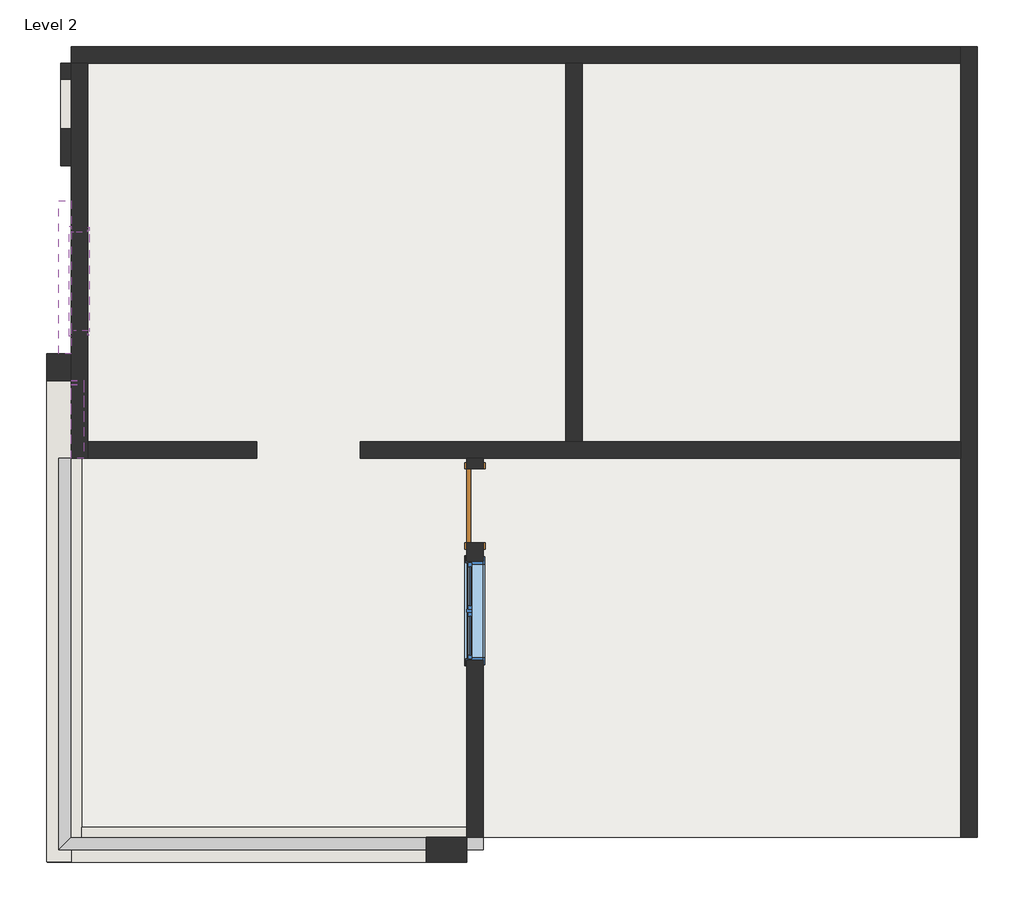
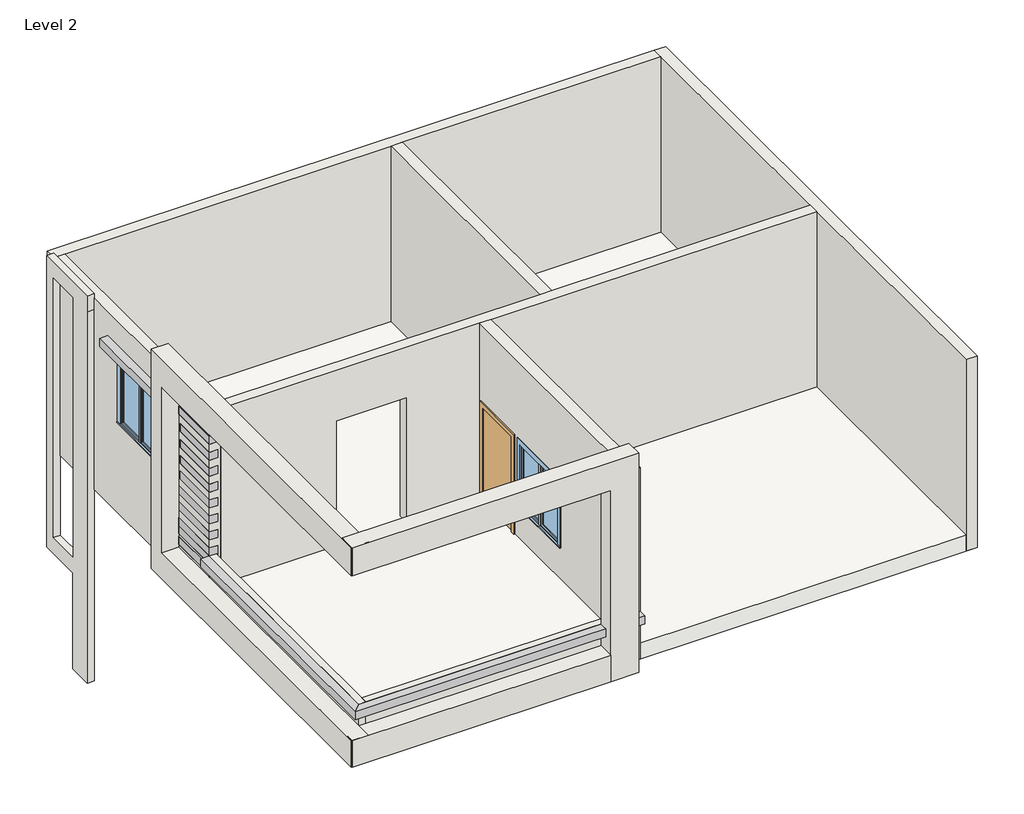
# One storey, incomplete: 14 proxies, 10 walls, 2 windows, 1 door, 1 roof.
"""IFC4 building model written with IfcOpenShell, lengths in millimetres."""

from ifc_helpers import new_model, si_unit, frame, origin, place, context, project, spatial, polyline, outline, extrude, faceted_brep, transform, mapped, element, save
from components import door_54dd4da4, walls_1_walls_1_33573b5d, window_0862ab64

model = new_model("IFC4")

# Units and contexts
model_context = context("Model", 3, world=origin())
ifc_project = project(units=[si_unit("LENGTHUNIT", "METRE", prefix="MILLI")], contexts=[model_context])

# Site, building, storey
site = spatial("IfcSite", under=ifc_project)
building = spatial("IfcBuilding", under=site)
storey = spatial("IfcBuildingStorey", under=building, Name="Level 2", Elevation=3657.6)

# Proxies
placement = place(None, origin())
element("IfcBuildingElementProxy", 1, Name="Cornice", ObjectType="Cornice", at=placement, inside=storey, context=model_context, shape_type="SweptSolid", body=[
    extrude(outline(polyline([(-12556.4681702, 5517.1742715), (-12708.8681702, 5517.1742715), (-12708.8681702, 7399.8573992), (-12556.4681702, 7399.8573992), (-12556.4681702, 5517.1742715)])), frame((0.0, 0.0, 6705.6), z_axis=(0.0, 0.0, 1.0), x_axis=(1.0, 0.0, 0.0)), (0.0, 0.0, 1.0), 152.4),
])
element("IfcBuildingElementProxy", 2, Name="Cornice", ObjectType="Cornice", at=placement, inside=storey, context=model_context, shape_type="SweptSolid", body=[
    extrude(outline(polyline([(-12708.8681702, 4224.2612165), (-12556.4681702, 4224.2612165), (-12556.4681702, -449.3387835), (-12708.8681702, -601.7387835), (-12708.8681702, 4224.2612165)])), frame((0.0, 0.0, 4419.6), z_axis=(0.0, 0.0, 1.0), x_axis=(1.0, 0.0, 0.0)), (0.0, 0.0, 1.0), 152.4),
])
element("IfcBuildingElementProxy", 3, Name="Cornice", ObjectType="Cornice", at=placement, inside=storey, context=model_context, shape_type="SweptSolid", body=[
    extrude(outline(polyline([(-12708.8681702, -601.7387835), (-12556.4681702, -449.3387835), (-7476.4681702, -449.3387835), (-7476.4681702, -601.7387835), (-12708.8681702, -601.7387835)])), frame((0.0, 0.0, 4419.6), z_axis=(0.0, 0.0, 1.0), x_axis=(1.0, 0.0, 0.0)), (0.0, 0.0, 1.0), 152.4),
])
element("IfcBuildingElementProxy", 4, Name="Reveal", ObjectType="Reveal", at=placement, inside=storey, context=model_context, shape_type="SweptSolid", body=[
    extrude(outline(polyline([(-12404.0681702, 4224.2612165), (-12556.4681702, 4224.2612165), (-12556.4681702, 5180.9930334), (-12404.0681702, 5180.9930334), (-12404.0681702, 4224.2612165)])), frame((0.0, 0.0, 7010.4), z_axis=(0.0, 0.0, 1.0), x_axis=(1.0, 0.0, 0.0)), (0.0, 0.0, 1.0), 152.4),
])
element("IfcBuildingElementProxy", 5, Name="Reveal", ObjectType="Reveal", at=placement, inside=storey, context=model_context, shape_type="SweptSolid", body=[
    extrude(outline(polyline([(-12404.0681702, 4224.2612165), (-12556.4681702, 4224.2612165), (-12556.4681702, 5180.9930334), (-12404.0681702, 5180.9930334), (-12404.0681702, 4224.2612165)])), frame((0.0, 0.0, 6705.6), z_axis=(0.0, 0.0, 1.0), x_axis=(1.0, 0.0, 0.0)), (0.0, 0.0, 1.0), 152.4),
])
element("IfcBuildingElementProxy", 6, Name="Reveal", ObjectType="Reveal", at=placement, inside=storey, context=model_context, shape_type="SweptSolid", body=[
    extrude(outline(polyline([(-12404.0681702, 4224.2612165), (-12556.4681702, 4224.2612165), (-12556.4681702, 5130.1930334), (-12404.0681702, 5130.1930334), (-12404.0681702, 4224.2612165)])), frame((0.0, 0.0, 6400.8), z_axis=(0.0, 0.0, 1.0), x_axis=(1.0, 0.0, 0.0)), (0.0, 0.0, 1.0), 152.4),
])
element("IfcBuildingElementProxy", 7, Name="Reveal", ObjectType="Reveal", at=placement, inside=storey, context=model_context, shape_type="SweptSolid", body=[
    extrude(outline(polyline([(-12404.0681702, 4224.2612165), (-12556.4681702, 4224.2612165), (-12556.4681702, 5130.1930334), (-12404.0681702, 5130.1930334), (-12404.0681702, 4224.2612165)])), frame((0.0, 0.0, 6096.0), z_axis=(0.0, 0.0, 1.0), x_axis=(1.0, 0.0, 0.0)), (0.0, 0.0, 1.0), 152.4),
])
element("IfcBuildingElementProxy", 8, Name="Reveal", ObjectType="Reveal", at=placement, inside=storey, context=model_context, shape_type="SweptSolid", body=[
    extrude(outline(polyline([(-12404.0681702, 4224.2612165), (-12556.4681702, 4224.2612165), (-12556.4681702, 5130.1930334), (-12404.0681702, 5130.1930334), (-12404.0681702, 4224.2612165)])), frame((0.0, 0.0, 5791.2), z_axis=(0.0, 0.0, 1.0), x_axis=(1.0, 0.0, 0.0)), (0.0, 0.0, 1.0), 152.4),
])
element("IfcBuildingElementProxy", 9, Name="Reveal", ObjectType="Reveal", at=placement, inside=storey, context=model_context, shape_type="SweptSolid", body=[
    extrude(outline(polyline([(-12404.0681702, 4224.2612165), (-12556.4681702, 4224.2612165), (-12556.4681702, 5138.6612165), (-12404.0681702, 5138.6612165), (-12404.0681702, 4224.2612165)])), frame((0.0, 0.0, 5486.4), z_axis=(0.0, 0.0, 1.0), x_axis=(1.0, 0.0, 0.0)), (0.0, 0.0, 1.0), 152.4),
])
element("IfcBuildingElementProxy", 10, Name="Reveal", ObjectType="Reveal", at=placement, inside=storey, context=model_context, shape_type="SweptSolid", body=[
    extrude(outline(polyline([(-12404.0681702, 4224.2612165), (-12556.4681702, 4224.2612165), (-12556.4681702, 5189.4612165), (-12404.0681702, 5189.4612165), (-12404.0681702, 4224.2612165)])), frame((0.0, 0.0, 5181.6), z_axis=(0.0, 0.0, 1.0), x_axis=(1.0, 0.0, 0.0)), (0.0, 0.0, 1.0), 152.4),
])
element("IfcBuildingElementProxy", 11, Name="Reveal", ObjectType="Reveal", at=placement, inside=storey, context=model_context, shape_type="SweptSolid", body=[
    extrude(outline(polyline([(-12404.0681702, 4224.2612165), (-12556.4681702, 4224.2612165), (-12556.4681702, 5189.4612165), (-12404.0681702, 5189.4612165), (-12404.0681702, 4224.2612165)])), frame((0.0, 0.0, 4876.8), z_axis=(0.0, 0.0, 1.0), x_axis=(1.0, 0.0, 0.0)), (0.0, 0.0, 1.0), 152.4),
])
element("IfcBuildingElementProxy", 12, Name="Reveal", ObjectType="Reveal", at=placement, inside=storey, context=model_context, shape_type="SweptSolid", body=[
    extrude(outline(polyline([(-12404.0681702, 4224.2612165), (-12556.4681702, 4224.2612165), (-12556.4681702, 5180.9930334), (-12404.0681702, 5180.9930334), (-12404.0681702, 4224.2612165)])), frame((0.0, 0.0, 4572.0), z_axis=(0.0, 0.0, 1.0), x_axis=(1.0, 0.0, 0.0)), (0.0, 0.0, 1.0), 152.4),
])
element("IfcBuildingElementProxy", 13, Name="Reveal", ObjectType="Reveal", at=placement, inside=storey, context=model_context, shape_type="SweptSolid", body=[
    extrude(outline(polyline([(-12404.0681702, 4224.2612165), (-12556.4681702, 4224.2612165), (-12556.4681702, 5180.9930334), (-12404.0681702, 5180.9930334), (-12404.0681702, 4224.2612165)])), frame((0.0, 0.0, 4419.6), z_axis=(0.0, 0.0, 1.0), x_axis=(1.0, 0.0, 0.0)), (0.0, 0.0, 1.0), 152.4),
])
element("IfcBuildingElementProxy", 14, Name="Reveal", ObjectType="Reveal", at=placement, inside=storey, context=model_context, shape_type="SweptSolid", body=[
    extrude(outline(polyline([(-12404.0681702, 4224.2612165), (-12556.4681702, 4224.2612165), (-12556.4681702, 5180.9930334), (-12404.0681702, 5180.9930334), (-12404.0681702, 4224.2612165)])), frame((0.0, 0.0, 4216.4), z_axis=(0.0, 0.0, 1.0), x_axis=(1.0, 0.0, 0.0)), (0.0, 0.0, 1.0), 152.4),
])

# Door
door_shape = door_54dd4da4(model_context)
element("IfcDoor", 15, ObjectType="Single-Flush : 36\" x 84\"", at=placement, inside=storey, context=model_context, shape_type="MappedRepresentation", body=[
    mapped(door_shape, transform((-7578.0681702, 3640.0612165, 3657.6), x_axis=(0.0, 1.0, 0.0), y_axis=(-1.0, 0.0, 0.0), z_axis=(0.0, 0.0, 1.0))),
])

# Roof
element("IfcRoof", 16, ObjectType="Generic - 12\"", at=placement, inside=storey, context=model_context, shape_type="SweptSolid", body=[
    extrude(outline(polyline([(-12556.4681702, 9304.2612165), (-1380.4681702, 9304.2612165), (-1380.4681702, -449.3387835), (-12556.4681702, -449.3387835), (-12556.4681702, 9304.2612165)])), frame((0.0, 0.0, 3657.6), z_axis=(0.0, 0.0, 1.0), x_axis=(1.0, 0.0, 0.0)), (0.0, 0.0, 1.0), 304.8),
])

# Walls
element("IfcWall", 17, ObjectType="Generic - 5\"", at=placement, inside=storey, context=model_context, shape_type="Brep", body=[
    faceted_brep([(-12556.4681702, 4224.2612165, 3962.4), (-12556.4681702, -449.3387835, 3962.4), (-12556.4681702, -449.3387835, 4572.0), (-12556.4681702, 4224.2612165, 4572.0), (-12556.4681702, 4224.2612165, 4419.6), (-12556.4681702, 4224.2612165, 4368.8), (-12556.4681702, 4224.2612165, 4216.4), (-12429.4681702, 4224.2612165, 3962.4), (-12429.4681702, 4224.2612165, 4572.0), (-12429.4681702, -322.3387835, 4572.0), (-12429.4681702, -449.3387835, 4572.0), (-12429.4681702, -449.3387835, 3962.4), (-12429.4681702, -322.3387835, 3962.4)], [[[0, 1, 2, 3, 4, 5, 6]], [[7, 8, 9, 10, 11, 12]], [[1, 0, 7, 12, 11]], [[3, 2, 10, 9, 8]], [[0, 6, 5, 4, 3, 8, 7]], [[2, 1, 11, 10]]]),
])
element("IfcWall", 18, ObjectType="Generic - 5\"", at=placement, inside=storey, context=model_context, shape_type="Brep", body=[
    faceted_brep([(-12429.4681702, -449.3387835, 3962.4), (-7679.6681702, -449.3387835, 3962.4), (-7679.6681702, -449.3387835, 4419.6), (-7679.6681702, -449.3387835, 4572.0), (-12429.4681702, -449.3387835, 4572.0), (-12429.4681702, -449.3387835, 4419.6), (-7679.6681702, -322.3387835, 3962.4), (-12429.4681702, -322.3387835, 3962.4), (-12429.4681702, -322.3387835, 4572.0), (-7679.6681702, -322.3387835, 4572.0)], [[[0, 1, 2, 3, 4, 5]], [[6, 7, 8, 9]], [[1, 0, 7, 6]], [[4, 3, 9, 8]], [[4, 8, 7, 0, 5]], [[1, 6, 9, 3, 2]]]),
])
element("IfcWall", 19, ObjectType="Generic - 5\"", at=placement, inside=storey, context=model_context, shape_type="SweptSolid", body=[
    extrude(outline(polyline([(7831.0612165, 0.0), (7831.0612165, 7094.0468042), (7831.0612165, 7398.8468042), (9101.0612165, 7398.8468042), (9101.0612165, 1828.8), (8288.2612165, 1828.8), (8288.2612165, 0.0), (7831.0612165, 0.0)]), holes=[polyline([(8897.8612165, 2133.6), (8897.8612165, 7094.0468042), (8288.2612165, 7094.0468042), (8288.2612165, 2133.6), (8897.8612165, 2133.6)])]), frame((-12683.4681702, 0.0, 0.0), z_axis=(1.0, 0.0, 0.0), x_axis=(0.0, 1.0, 0.0)), (0.0, 0.0, 1.0), 127.0),
])
element("IfcWall", 20, ObjectType="Generic - 8\"", at=placement, inside=storey, context=model_context, shape_type="Brep", body=[
    faceted_brep([(-12556.4681702, 9101.0612165, 3657.6), (-12353.2681702, 9101.0612165, 3657.6), (-6460.4681702, 9101.0612165, 3657.6), (-6257.2681702, 9101.0612165, 3657.6), (-1583.6681702, 9101.0612165, 3657.6), (-1583.6681702, 9101.0612165, 7315.2), (-6257.2681702, 9101.0612165, 7315.2), (-6460.4681702, 9101.0612165, 7315.2), (-12353.2681702, 9101.0612165, 7315.2), (-12556.4681702, 9101.0612165, 7315.2), (-12556.4681702, 9304.2612165, 3657.6), (-12556.4681702, 9304.2612165, 7315.2), (-1583.6681702, 9304.2612165, 7315.2), (-1583.6681702, 9304.2612165, 3657.6)], [[[0, 1, 2, 3, 4, 5, 6, 7, 8, 9]], [[10, 11, 12, 13]], [[4, 3, 2, 1, 0, 10, 13]], [[9, 8, 7, 6, 5, 12, 11]], [[0, 9, 11, 10]], [[5, 4, 13, 12]]]),
])
element("IfcWall", 21, ObjectType="Generic - 8\"", at=placement, inside=storey, context=model_context, shape_type="Brep", body=[
    faceted_brep([(-12353.2681702, 4224.2612165, 3657.6), (-12353.2681702, 4427.4612165, 3657.6), (-12353.2681702, 9101.0612165, 3657.6), (-12353.2681702, 9101.0612165, 7315.2), (-12353.2681702, 4427.4612165, 7315.2), (-12353.2681702, 4224.2612165, 7315.2), (-12353.2681702, 7018.2612165, 6617.6597463), (-12353.2681702, 7018.2612165, 5398.4597463), (-12353.2681702, 5799.0612165, 5398.4597463), (-12353.2681702, 5799.0612165, 6617.6597463), (-12556.4681702, 9101.0612165, 3657.6), (-12556.4681702, 4224.2612165, 3657.6), (-12556.4681702, 4224.2612165, 3962.4), (-12556.4681702, 4224.2612165, 4216.4), (-12556.4681702, 5180.9930334, 4216.4), (-12556.4681702, 5180.9930334, 4368.8), (-12556.4681702, 4224.2612165, 4368.8), (-12556.4681702, 4224.2612165, 4419.6), (-12556.4681702, 5180.9930334, 4419.6), (-12556.4681702, 5180.9930334, 4724.4), (-12556.4681702, 4224.2612165, 4724.4), (-12556.4681702, 4224.2612165, 4876.8), (-12556.4681702, 5189.4612165, 4876.8), (-12556.4681702, 5189.4612165, 5029.2), (-12556.4681702, 4224.2612165, 5029.2), (-12556.4681702, 4224.2612165, 5181.6), (-12556.4681702, 5189.4612165, 5181.6), (-12556.4681702, 5189.4612165, 5334.0), (-12556.4681702, 4224.2612165, 5334.0), (-12556.4681702, 4224.2612165, 5486.4), (-12556.4681702, 5138.6612165, 5486.4), (-12556.4681702, 5138.6612165, 5638.8), (-12556.4681702, 4224.2612165, 5638.8), (-12556.4681702, 4224.2612165, 5791.2), (-12556.4681702, 5130.1930334, 5791.2), (-12556.4681702, 5130.1930334, 5943.6), (-12556.4681702, 4224.2612165, 5943.6), (-12556.4681702, 4224.2612165, 6096.0), (-12556.4681702, 5130.1930334, 6096.0), (-12556.4681702, 5130.1930334, 6248.4), (-12556.4681702, 4224.2612165, 6248.4), (-12556.4681702, 4224.2612165, 6400.8), (-12556.4681702, 5130.1930334, 6400.8), (-12556.4681702, 5130.1930334, 6553.2), (-12556.4681702, 4224.2612165, 6553.2), (-12556.4681702, 4224.2612165, 6705.6), (-12556.4681702, 5180.9930334, 6705.6), (-12556.4681702, 5180.9930334, 6858.0), (-12556.4681702, 4224.2612165, 6858.0), (-12556.4681702, 4224.2612165, 7010.4), (-12556.4681702, 5180.9930334, 7010.4), (-12556.4681702, 5180.9930334, 7162.8), (-12556.4681702, 4224.2612165, 7162.8), (-12556.4681702, 4224.2612165, 7315.2), (-12556.4681702, 9101.0612165, 7315.2), (-12556.4681702, 7018.2612165, 5398.4597463), (-12556.4681702, 7018.2612165, 6617.6597463), (-12556.4681702, 5799.0612165, 6617.6597463), (-12556.4681702, 5799.0612165, 5398.4597463), (-12404.0681702, 4224.2612165, 7162.8), (-12404.0681702, 4224.2612165, 7010.4), (-12404.0681702, 4224.2612165, 6858.0), (-12404.0681702, 4224.2612165, 6705.6), (-12404.0681702, 4224.2612165, 6553.2), (-12404.0681702, 4224.2612165, 6400.8), (-12404.0681702, 4224.2612165, 6248.4), (-12404.0681702, 4224.2612165, 6096.0), (-12404.0681702, 4224.2612165, 5943.6), (-12404.0681702, 4224.2612165, 5791.2), (-12404.0681702, 4224.2612165, 5638.8), (-12404.0681702, 4224.2612165, 5486.4), (-12404.0681702, 4224.2612165, 5334.0), (-12404.0681702, 4224.2612165, 5181.6), (-12404.0681702, 4224.2612165, 5029.2), (-12404.0681702, 4224.2612165, 4876.8), (-12404.0681702, 4224.2612165, 4724.4), (-12404.0681702, 4224.2612165, 4419.6), (-12404.0681702, 4224.2612165, 4368.8), (-12404.0681702, 4224.2612165, 4216.4), (-12404.0681702, 5180.9930334, 7010.4), (-12404.0681702, 5180.9930334, 7162.8), (-12404.0681702, 5180.9930334, 6705.6), (-12404.0681702, 5180.9930334, 6858.0), (-12404.0681702, 5189.4612165, 5181.6), (-12404.0681702, 5189.4612165, 5334.0), (-12404.0681702, 5189.4612165, 4876.8), (-12404.0681702, 5189.4612165, 5029.2), (-12404.0681702, 5180.9930334, 4724.4), (-12404.0681702, 5180.9930334, 4419.6), (-12404.0681702, 5180.9930334, 4216.4), (-12404.0681702, 5180.9930334, 4368.8), (-12404.0681702, 5130.1930334, 6553.2), (-12404.0681702, 5130.1930334, 6400.8), (-12404.0681702, 5130.1930334, 6248.4), (-12404.0681702, 5130.1930334, 6096.0), (-12404.0681702, 5130.1930334, 5943.6), (-12404.0681702, 5130.1930334, 5791.2), (-12404.0681702, 5138.6612165, 5638.8), (-12404.0681702, 5138.6612165, 5486.4)], [[[0, 1, 2, 3, 4, 5], [6, 7, 8, 9]], [[10, 11, 12, 13, 14, 15, 16, 17, 18, 19, 20, 21, 22, 23, 24, 25, 26, 27, 28, 29, 30, 31, 32, 33, 34, 35, 36, 37, 38, 39, 40, 41, 42, 43, 44, 45, 46, 47, 48, 49, 50, 51, 52, 53, 54], [55, 56, 57, 58]], [[2, 1, 0, 11, 10]], [[5, 4, 3, 54, 53]], [[3, 2, 10, 54]], [[5, 53, 52, 59, 60, 49, 48, 61, 62, 45, 44, 63, 64, 41, 40, 65, 66, 37, 36, 67, 68, 33, 32, 69, 70, 29, 28, 71, 72, 25, 24, 73, 74, 21, 20, 75, 76, 17, 16, 77, 78, 13, 12, 11, 0]], [[79, 50, 49, 60]], [[79, 60, 59, 80]], [[80, 59, 52, 51]], [[81, 46, 45, 62]], [[81, 62, 61, 82]], [[82, 61, 48, 47]], [[83, 26, 25, 72]], [[83, 72, 71, 84]], [[84, 71, 28, 27]], [[85, 22, 21, 74]], [[85, 74, 73, 86]], [[86, 73, 24, 23]], [[75, 87, 88, 76]], [[87, 75, 20, 19]], [[88, 18, 17, 76]], [[89, 14, 13, 78]], [[90, 89, 78, 77]], [[15, 90, 77, 16]], [[90, 15, 14, 89]], [[87, 19, 18, 88]], [[22, 85, 86, 23]], [[26, 83, 84, 27]], [[46, 81, 82, 47]], [[50, 79, 80, 51]], [[7, 6, 56, 55]], [[8, 7, 55, 58]], [[9, 8, 58, 57]], [[6, 9, 57, 56]], [[91, 43, 42, 92]], [[92, 42, 41, 64]], [[91, 92, 64, 63]], [[43, 91, 63, 44]], [[93, 39, 38, 94]], [[94, 38, 37, 66]], [[93, 94, 66, 65]], [[39, 93, 65, 40]], [[95, 35, 34, 96]], [[96, 34, 33, 68]], [[95, 96, 68, 67]], [[35, 95, 67, 36]], [[97, 31, 30, 98]], [[98, 30, 29, 70]], [[97, 98, 70, 69]], [[31, 97, 69, 32]]]),
])
element("IfcWall", 22, ObjectType="Generic - 8\"", at=placement, inside=storey, context=model_context, shape_type="Brep", body=[
    faceted_brep([(-1583.6681702, 9304.2612165, 3657.6), (-1583.6681702, 9101.0612165, 3657.6), (-1583.6681702, 4427.4612165, 3657.6), (-1583.6681702, 4224.2612165, 3657.6), (-1583.6681702, -449.3387835, 3657.6), (-1583.6681702, -449.3387835, 7315.2), (-1583.6681702, 4224.2612165, 7315.2), (-1583.6681702, 4427.4612165, 7315.2), (-1583.6681702, 9101.0612165, 7315.2), (-1583.6681702, 9304.2612165, 7315.2), (-1380.4681702, 9304.2612165, 3657.6), (-1380.4681702, 9304.2612165, 7315.2), (-1380.4681702, -449.3387835, 7315.2), (-1380.4681702, -449.3387835, 3657.6)], [[[0, 1, 2, 3, 4, 5, 6, 7, 8, 9]], [[10, 11, 12, 13]], [[4, 3, 2, 1, 0, 10, 13]], [[9, 8, 7, 6, 5, 12, 11]], [[0, 9, 11, 10]], [[4, 13, 12, 5]]]),
])
element("IfcWall", 23, ObjectType="Generic - 8\"", at=placement, inside=storey, context=model_context, shape_type="Brep", body=[
    faceted_brep([(-7679.6681702, 4224.2612165, 3657.6), (-7679.6681702, 4097.2612165, 3657.6), (-7679.6681702, 4097.2612165, 5791.2), (-7679.6681702, 3182.8612165, 5791.2), (-7679.6681702, 3182.8612165, 3657.6), (-7679.6681702, -449.3387835, 3657.6), (-7679.6681702, -449.3387835, 3962.4), (-7679.6681702, -449.3387835, 4572.0), (-7679.6681702, -449.3387835, 7315.2), (-7679.6681702, 2954.2612165, 7315.2), (-7679.6681702, 3868.6612165, 7315.2), (-7679.6681702, 4224.2612165, 7315.2), (-7679.6681702, 2954.2612165, 5791.2), (-7679.6681702, 1735.0612165, 5791.2), (-7679.6681702, 1735.0612165, 4572.0), (-7679.6681702, 2954.2612165, 4572.0), (-7476.4681702, 4097.2612165, 5791.2), (-7476.4681702, 4097.2612165, 3657.6), (-7476.4681702, 4224.2612165, 3657.6), (-7476.4681702, 4224.2612165, 7315.2), (-7476.4681702, 3868.6612165, 7315.2), (-7476.4681702, 2954.2612165, 7315.2), (-7476.4681702, -449.3387835, 7315.2), (-7476.4681702, -449.3387835, 3657.6), (-7476.4681702, 3182.8612165, 3657.6), (-7476.4681702, 3182.8612165, 5791.2), (-7476.4681702, 2954.2612165, 5791.2), (-7476.4681702, 2954.2612165, 4572.0), (-7476.4681702, 1735.0612165, 4572.0), (-7476.4681702, 1735.0612165, 5791.2)], [[[0, 1, 2, 3, 4, 5, 6, 7, 8, 9, 10, 11], [12, 13, 14, 15]], [[16, 17, 18, 19, 20, 21, 22, 23, 24, 25], [26, 27, 28, 29]], [[18, 17, 1, 0]], [[24, 23, 5, 4]], [[11, 10, 9, 8, 22, 21, 20, 19]], [[0, 11, 19, 18]], [[5, 23, 22, 8, 7, 6]], [[27, 26, 12, 15]], [[28, 27, 15, 14]], [[29, 28, 14, 13]], [[26, 29, 13, 12]], [[2, 1, 17, 16]], [[3, 2, 16, 25]], [[4, 3, 25, 24]]]),
])
element("IfcWall", 24, ObjectType="Generic - 8\"", at=placement, inside=storey, context=model_context, shape_type="Brep", body=[
    faceted_brep([(-12353.2681702, 4224.2612165, 7315.2), (-12353.2681702, 4224.2612165, 3657.6), (-10267.8388214, 4224.2612165, 3657.6), (-10267.8388214, 4224.2612165, 6351.2959794), (-8991.5303488, 4224.2612165, 6351.2959794), (-8991.5303488, 4224.2612165, 3657.6), (-7679.6681702, 4224.2612165, 3657.6), (-7476.4681702, 4224.2612165, 3657.6), (-1583.6681702, 4224.2612165, 3657.6), (-1583.6681702, 4224.2612165, 7315.2), (-7476.4681702, 4224.2612165, 7315.2), (-7679.6681702, 4224.2612165, 7315.2), (-12353.2681702, 4427.4612165, 3657.6), (-12353.2681702, 4427.4612165, 7315.2), (-6460.4681702, 4427.4612165, 7315.2), (-6257.2681702, 4427.4612165, 7315.2), (-1583.6681702, 4427.4612165, 7315.2), (-1583.6681702, 4427.4612165, 3657.6), (-6257.2681702, 4427.4612165, 3657.6), (-6460.4681702, 4427.4612165, 3657.6), (-8991.5303488, 4427.4612165, 3657.6), (-8991.5303488, 4427.4612165, 6351.2959794), (-10267.8388214, 4427.4612165, 6351.2959794), (-10267.8388214, 4427.4612165, 3657.6)], [[[0, 1, 2, 3, 4, 5, 6, 7, 8, 9, 10, 11]], [[12, 13, 14, 15, 16, 17, 18, 19, 20, 21, 22, 23]], [[9, 8, 17, 16]], [[0, 13, 12, 1]], [[0, 11, 10, 9, 16, 15, 14, 13]], [[5, 4, 21, 20]], [[3, 2, 23, 22]], [[4, 3, 22, 21]], [[2, 1, 12, 23]], [[8, 7, 6, 5, 20, 19, 18, 17]]]),
])
element("IfcWall", 25, ObjectType="Generic - 8\"", at=placement, inside=storey, context=model_context, shape_type="SweptSolid", body=[
    extrude(outline(polyline([(-6460.4681702, 4427.4612165), (-6460.4681702, 9101.0612165), (-6257.2681702, 9101.0612165), (-6257.2681702, 4427.4612165), (-6460.4681702, 4427.4612165)])), frame((0.0, 0.0, 3657.6), z_axis=(0.0, 0.0, 1.0), x_axis=(1.0, 0.0, 0.0)), (0.0, 0.0, 1.0), 3657.6),
])
walls_1_walls_1_shape = walls_1_walls_1_33573b5d(model_context)
element("IfcWall", 26, ObjectType="Walls 1 : Walls 1", at=placement, inside=storey, context=model_context, shape_type="MappedRepresentation", body=[
    mapped(walls_1_walls_1_shape, transform((0.0, 0.0, 0.0), x_axis=(1.0, 0.0, 0.0), y_axis=(0.0, 1.0, 0.0), z_axis=(0.0, 0.0, 1.0))),
])

# Windows
window_shape = window_0862ab64(model_context)
element("IfcWindow", 27, ObjectType="Casement Dbl with Trim : 48\" x 48\"", at=placement, inside=storey, context=model_context, shape_type="MappedRepresentation", body=[
    mapped(window_shape, transform((-12435.8181702, 6408.6612165, 4484.0597463), x_axis=(0.0, 1.0, 0.0), y_axis=(-1.0, 0.0, 0.0), z_axis=(0.0, 0.0, 1.0))),
])
element("IfcWindow", 28, ObjectType="Casement Dbl with Trim : 48\" x 48\"", at=placement, inside=storey, context=model_context, shape_type="MappedRepresentation", body=[
    mapped(window_shape, transform((-7559.0181702, 2344.6612165, 3657.6), x_axis=(0.0, 1.0, 0.0), y_axis=(-1.0, 0.0, 0.0), z_axis=(0.0, 0.0, 1.0))),
])

save(model, "model.ifc")

# Revit data of these elements
# Type "Single-Flush : 36\" x 84\""
#   Type Mark = "1"
#   Construction Type Id = "MDOOR"
#   Assembly Code = "C1020"
#   Analytic Construction = "Metal"
#   Thickness = 0' - 2"
#   Heat Transfer Coefficient (U) = 0.651978 BTU/(h·ft²·°F)
#   Height = 7' - 0"
#   Trim Projection Ext = 0' - 1"
#   Trim Projection Int = 0' - 1"
#   Trim Width = 0' - 3"
#   Width = 3' - 0"
#   Define Thermal Properties by = 1
#   Door Material = Door - Panel
#   Frame Material = Door - Frame
#   Visual Light Transmittance = 0
#   Solar Heat Gain Coefficient = 0
#   Function = (empty or 0)
#   Wall Closure = (empty or 0)
# Type "Generic - 12\""
#   Assembly Code = "B1020"
#   Layers, outside or top first: 1' - 0" no material (function 1)
# Type "Generic - 5\""
#   Assembly Code = "B2010"
#   Layers, outside or top first: 0' - 5" no material (function 1)
# Type "Generic - 8\""
#   Assembly Code = "B2010"
#   Layers, outside or top first: 0' - 8" no material (function 1)
# Type "Casement Dbl with Trim : 48\" x 48\""
#   Type Mark = "13"
#   Construction Type Id = "GSP4R"
#   Assembly Code = "B2020100"
#   Analytic Construction = "1/8 in Pilkington single glazing"
#   Visual Light Transmittance = 0.9
#   Solar Heat Gain Coefficient = 0.78
#   Heat Transfer Coefficient (U) = 0.6496 BTU/(h·ft²·°F)
#   Height = 4' - 0"
#   Default Sill Height = 3' - 0"
#   Trim Projection - Ext. = 0' - 0 1/2"
#   Trim Projection - Int. = 0' - 0 3/4"
#   Trim Width - Exterior = 0' - 3 1/2"
#   Trim Width - Interior = 0' - 3 1/2"
#   Width = 4' - 0"
#   Window Inset = 0' - 0 3/4"
#   Define Thermal Properties by = 1
#   Glass Pane Material = Glass
#   Sash Material = Sash
#   Trim Exterior Material = Trim
#   Trim Interior Material = Trim
#   Wall Closure = (empty or 0)
# Elements 1, 2, 3 (IfcBuildingElementProxy, "Cornice")
#   Phase Created = New Construction
#   Materials on its faces: "Default Wall"
# Element 15 (IfcDoor, "Single-Flush : 36\" x 84\"")
#   Phase Created = New Construction
#   Materials on its faces: "Door - Frame", "Door - Panel"
# Element 16 (IfcRoof, "Generic - 12\"")
#   built-in parameter 1001705 = 13 (stored number, unit not read)
#   built-in parameter 1001710 = 33615
#   Phase Created = New Construction
#   Materials on its faces: "Default Roof"
# Elements 17, 18 (IfcWall, "Generic - 5\"")
#   built-in parameter 1001111 = 1' - 0"
#   Top Offset = -9' - 0"
#   Base Offset = 1' - 0"
#   wall height = 2' - 0"
#   Phase Created = New Construction
#   Base Constraint = Level 2
#   Top Constraint = Level 3
#   Materials on its faces: "Default Wall"
# Element 19 (IfcWall, "Generic - 5\"")
#   built-in parameter 1001111 = -12' - 0"
#   Top Offset = -0' - 8.70682"
#   Base Offset = -12' - 0"
#   wall height = 23' - 3.29318"
#   Phase Created = New Construction
#   Base Constraint = Level 2
#   Top Constraint = Level 3
#   Materials on its faces: "Default Wall"
# Elements 20, 21, 22, 23, 24, 25 (IfcWall, "Generic - 8\"")
#   Top Offset = 0' - 0"
#   Base Offset = 0' - 0"
#   Unconnected Height = 12' - 0"
#   wall height = 12' - 0"
#   Phase Created = New Construction
#   Base Constraint = Level 2
#   Materials on its faces: "Default Wall"
# Element 26 (IfcWall, "Walls 1 : Walls 1")
#   Phase Created = New Construction
#   Materials on its faces: "Default Wall"
# Element 27 (IfcWindow, "Casement Dbl with Trim : 48\" x 48\"")
#   Mark = "2"
#   Phase Created = New Construction
#   Materials on its faces: "Sash", "Trim", "Glass"
# Element 28 (IfcWindow, "Casement Dbl with Trim : 48\" x 48\"")
#   Mark = "4"
#   Phase Created = New Construction
#   Materials on its faces: "Sash", "Trim", "Glass"
# Materials
#   "Door - Panel": class "Wood", colour RGB 210 159 95, transparency 0
#   "Door - Frame": colour RGB 118 70 51, transparency 0
#   "Glass": class "Glass", colour RGB 0 128 192, transparency 0.75, Description = "Soda Lime Glass", Cost = 0
#   "Sash": class "Wood", colour RGB 224 178 126, transparency 0
#   "Trim": class "Wood", colour RGB 224 178 126, transparency 0
#   "Default Wall": colour RGB 128 128 128, transparency 0
#   "Default Roof": colour RGB 88 101 114, transparency 0
